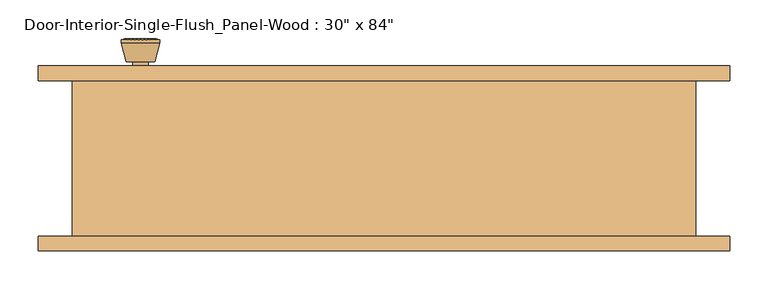
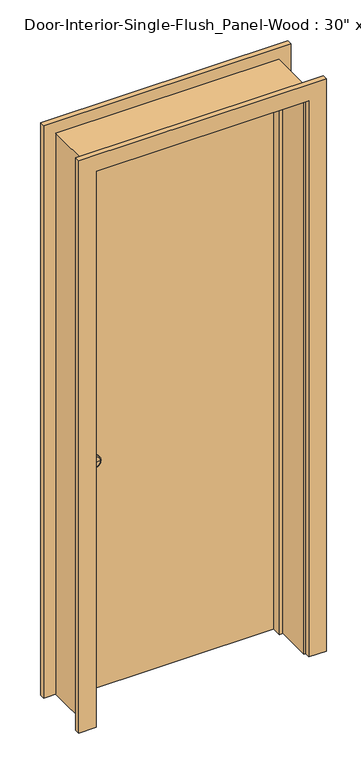
"""IFC4 building model written with IfcOpenShell, lengths in millimetres: door geometry."""

from ifc_helpers import new_model, si_unit, point, frame, frame_2d, origin, origin_with_axes, place, context, project, spatial, polyline, circle_curve, trimmed, segment, composite_curve, outline, extrude, faceted_brep, source, transform, mapped, element, save
from ifc_brep_helpers import plane_surface, cylinder_surface, revolved_surface, advanced_brep


def door_715cd483(model_context):
    return source(origin(), model_context, "Body", "SolidModel", [
        advanced_brep(
        [(-317.5, 57.5, 914.4), (-307.5, 57.5, 914.4), (-327.5, 57.5, 914.4), (-297.0241324, 8.5, 914.4), (-317.5, 8.5, 914.4), (-337.9758676, 8.5, 914.4), (-292.5, 10.3278681, 914.4), (-342.5, 10.3278681, 914.4), (-292.5, 13.7915463, 914.4), (-342.5, 13.7915463, 914.4), (-298.863764, 38.5, 914.4), (-336.136236, 38.5, 914.4), (-307.5, 38.5, 914.4), (-327.5, 38.5, 914.4)],
        [
            (0, 1),
            (1, 2, circle_curve(frame((-317.5, 57.5, 914.4), z_axis=(0.0, 1.0, 0.0), x_axis=(-1.0, 0.0, 0.0)), 10.0)),
            (2, 0),
            (2, 1, circle_curve(frame((-317.5, 57.5, 914.4), z_axis=(0.0, 1.0, 0.0), x_axis=(-1.0, 0.0, 0.0)), 10.0)),
            (3, 4),
            (4, 5),
            (5, 3, circle_curve(frame((-317.5, 8.5, 914.4), z_axis=(0.0, -1.0, 0.0), x_axis=(-1.0, 0.0, 0.0)), 20.4758676)),
            (3, 5, circle_curve(frame((-317.5, 8.5, 914.4), z_axis=(0.0, -1.0, 0.0), x_axis=(-1.0, 0.0, 0.0)), 20.4758676)),
            (6, 3),
            (5, 7),
            (7, 6, circle_curve(frame((-317.5, 10.3278681, 914.4), z_axis=(0.0, -1.0, 0.0), x_axis=(-1.0, 0.0, 0.0)), 25.0)),
            (6, 7, circle_curve(frame((-317.5, 10.3278681, 914.4), z_axis=(0.0, -1.0, 0.0), x_axis=(-1.0, 0.0, 0.0)), 25.0)),
            (8, 6),
            (7, 9),
            (9, 8, circle_curve(frame((-317.5, 13.7915463, 914.4), z_axis=(0.0, -1.0, 0.0), x_axis=(-1.0, 0.0, 0.0)), 25.0)),
            (8, 9, circle_curve(frame((-317.5, 13.7915463, 914.4), z_axis=(0.0, -1.0, 0.0), x_axis=(-1.0, 0.0, 0.0)), 25.0)),
            (10, 8),
            (9, 11),
            (11, 10, circle_curve(frame((-317.5, 38.5, 914.4), z_axis=(0.0, -1.0, 0.0), x_axis=(-1.0, 0.0, 0.0)), 18.636236)),
            (10, 11, circle_curve(frame((-317.5, 38.5, 914.4), z_axis=(0.0, -1.0, 0.0), x_axis=(-1.0, 0.0, 0.0)), 18.636236)),
            (12, 10),
            (11, 13),
            (13, 12, circle_curve(frame((-317.5, 38.5, 914.4), z_axis=(0.0, -1.0, 0.0), x_axis=(-1.0, 0.0, 0.0)), 10.0)),
            (12, 13, circle_curve(frame((-317.5, 38.5, 914.4), z_axis=(0.0, -1.0, 0.0), x_axis=(-1.0, 0.0, 0.0)), 10.0)),
            (1, 12),
            (13, 2),
        ],
        [
            plane_surface(frame((-317.5, 57.5, 914.4), z_axis=(0.0, 1.0, 0.0), x_axis=(-1.0, 0.0, 0.0))),
            plane_surface(frame((-317.5, 8.5, 914.4), z_axis=(0.0, -1.0, 0.0), x_axis=(-1.0, 0.0, 0.0))),
            revolved_surface(polyline([(-337.9758676, 8.5, 914.4), (-342.5, 10.3278681, 914.4)]), (-317.5, 57.5, 914.4), (0.0, 1.0, 0.0)),
            cylinder_surface(frame((-317.5, 57.5, 914.4), z_axis=(0.0, 1.0, 0.0), x_axis=(-1.0, 0.0, 0.0)), 25.0),
            revolved_surface(polyline([(-342.5, 13.7915463, 914.4), (-336.136236, 38.5, 914.4)]), (-317.5, 57.5, 914.4), (0.0, 1.0, 0.0)),
            plane_surface(frame((-317.5, 38.5, 914.4), z_axis=(0.0, 1.0, 0.0), x_axis=(-1.0, 0.0, 0.0))),
            cylinder_surface(frame((-317.5, 57.5, 914.4), z_axis=(0.0, 1.0, 0.0), x_axis=(-1.0, 0.0, 0.0)), 10.0),
        ],
        [
            (0, [[1, 2, 3]]),
            (0, [[-3, 4, -1]]),
            (1, [[5, 6, 7]]),
            (1, [[-6, -5, 8]]),
            (2, [[9, -7, 10, 11]]),
            (2, [[-10, -8, -9, 12]]),
            (3, [[13, -11, 14, 15]]),
            (3, [[-14, -12, -13, 16]]),
            (4, [[17, -15, 18, 19]]),
            (4, [[-18, -16, -17, 20]]),
            (5, [[21, -19, 22, 23]]),
            (5, [[-22, -20, -21, 24]]),
            (6, [[25, -23, 26, -2]]),
            (6, [[-26, -24, -25, -4]]),
        ],
    ),
        extrude(outline(composite_curve([segment(trimmed(circle_curve(frame_2d((914.4, -317.5)), 30.0), [point((914.4, -347.5))], [point((914.4, -287.5))], False, "CARTESIAN"), True, "CONTINUOUS"), segment(trimmed(circle_curve(frame_2d((914.4, -317.5)), 30.0), [point((914.4, -287.5))], [point((914.4, -347.5))], False, "CARTESIAN"), True, "CONTINUOUS")], self_intersect=False)), frame((0.0, 57.5, 0.0), z_axis=(0.0, 1.0, 0.0), x_axis=(0.0, 0.0, 1.0)), (0.0, 0.0, 1.0), 6.0),
        advanced_brep(
        [(-317.5, 104.425, 914.4), (-327.5, 104.425, 914.4), (-307.5, 104.425, 914.4), (-297.0241324, 153.425, 914.4), (-337.9758676, 153.425, 914.4), (-317.5, 153.425, 914.4), (-292.5, 151.5971319, 914.4), (-342.5, 151.5971319, 914.4), (-292.5, 148.1334537, 914.4), (-342.5, 148.1334537, 914.4), (-298.863764, 123.425, 914.4), (-336.136236, 123.425, 914.4), (-307.5, 123.425, 914.4), (-327.5, 123.425, 914.4)],
        [
            (0, 1),
            (1, 2, circle_curve(frame((-317.5, 104.425, 914.4), z_axis=(0.0, -1.0, 0.0), x_axis=(-1.0, 0.0, 0.0)), 10.0)),
            (2, 0),
            (2, 1, circle_curve(frame((-317.5, 104.425, 914.4), z_axis=(0.0, -1.0, 0.0), x_axis=(-1.0, 0.0, 0.0)), 10.0)),
            (3, 4, circle_curve(frame((-317.5, 153.425, 914.4), z_axis=(0.0, 1.0, 0.0), x_axis=(-1.0, 0.0, 0.0)), 20.4758676)),
            (4, 5),
            (5, 3),
            (4, 3, circle_curve(frame((-317.5, 153.425, 914.4), z_axis=(0.0, 1.0, 0.0), x_axis=(-1.0, 0.0, 0.0)), 20.4758676)),
            (6, 7, circle_curve(frame((-317.5, 151.5971319, 914.4), z_axis=(0.0, 1.0, 0.0), x_axis=(-1.0, 0.0, 0.0)), 25.0)),
            (7, 4),
            (3, 6),
            (7, 6, circle_curve(frame((-317.5, 151.5971319, 914.4), z_axis=(0.0, 1.0, 0.0), x_axis=(-1.0, 0.0, 0.0)), 25.0)),
            (8, 9, circle_curve(frame((-317.5, 148.1334537, 914.4), z_axis=(0.0, 1.0, 0.0), x_axis=(-1.0, 0.0, 0.0)), 25.0)),
            (9, 7),
            (6, 8),
            (9, 8, circle_curve(frame((-317.5, 148.1334537, 914.4), z_axis=(0.0, 1.0, 0.0), x_axis=(-1.0, 0.0, 0.0)), 25.0)),
            (10, 11, circle_curve(frame((-317.5, 123.425, 914.4), z_axis=(0.0, 1.0, 0.0), x_axis=(-1.0, 0.0, 0.0)), 18.636236)),
            (11, 9),
            (8, 10),
            (11, 10, circle_curve(frame((-317.5, 123.425, 914.4), z_axis=(0.0, 1.0, 0.0), x_axis=(-1.0, 0.0, 0.0)), 18.636236)),
            (12, 13, circle_curve(frame((-317.5, 123.425, 914.4), z_axis=(0.0, 1.0, 0.0), x_axis=(-1.0, 0.0, 0.0)), 10.0)),
            (13, 11),
            (10, 12),
            (13, 12, circle_curve(frame((-317.5, 123.425, 914.4), z_axis=(0.0, 1.0, 0.0), x_axis=(-1.0, 0.0, 0.0)), 10.0)),
            (1, 13),
            (12, 2),
        ],
        [
            plane_surface(frame((-317.5, 104.425, 914.4), z_axis=(0.0, -1.0, 0.0), x_axis=(-1.0, 0.0, 0.0))),
            plane_surface(frame((-317.5, 153.425, 914.4), z_axis=(0.0, 1.0, 0.0), x_axis=(-1.0, 0.0, 0.0))),
            revolved_surface(polyline([(-337.9758676, 153.425, 914.4), (-342.5, 151.5971319, 914.4)]), (-317.5, 104.425, 914.4), (0.0, -1.0, 0.0)),
            cylinder_surface(frame((-317.5, 104.425, 914.4), z_axis=(0.0, -1.0, 0.0), x_axis=(-1.0, 0.0, 0.0)), 25.0),
            revolved_surface(polyline([(-342.5, 148.1334537, 914.4), (-336.136236, 123.425, 914.4)]), (-317.5, 104.425, 914.4), (0.0, -1.0, 0.0)),
            plane_surface(frame((-317.5, 123.425, 914.4), z_axis=(0.0, -1.0, 0.0), x_axis=(-1.0, 0.0, 0.0))),
            cylinder_surface(frame((-317.5, 104.425, 914.4), z_axis=(0.0, -1.0, 0.0), x_axis=(-1.0, 0.0, 0.0)), 10.0),
        ],
        [
            (0, [[1, 2, 3]]),
            (0, [[-3, 4, -1]]),
            (1, [[5, 6, 7]]),
            (1, [[8, -7, -6]]),
            (2, [[9, 10, -5, 11]]),
            (2, [[12, -11, -8, -10]]),
            (3, [[13, 14, -9, 15]]),
            (3, [[16, -15, -12, -14]]),
            (4, [[17, 18, -13, 19]]),
            (4, [[20, -19, -16, -18]]),
            (5, [[21, 22, -17, 23]]),
            (5, [[24, -23, -20, -22]]),
            (6, [[-2, 25, -21, 26]]),
            (6, [[-4, -26, -24, -25]]),
        ],
    ),
        extrude(outline(composite_curve([segment(trimmed(circle_curve(frame_2d((914.4, -317.5)), 30.0), [point((914.4, -347.5))], [point((914.4, -287.5))], False, "CARTESIAN"), True, "CONTINUOUS"), segment(trimmed(circle_curve(frame_2d((914.4, -317.5)), 30.0), [point((914.4, -287.5))], [point((914.4, -347.5))], False, "CARTESIAN"), True, "CONTINUOUS")], self_intersect=False)), frame((0.0, 98.425, 0.0), z_axis=(0.0, 1.0, 0.0), x_axis=(0.0, 0.0, 1.0)), (0.0, 0.0, 1.0), 6.0),
        extrude(outline(polyline([(381.0, 63.5), (-381.0, 63.5), (-381.0, 98.425), (381.0, 98.425), (381.0, 63.5)])), origin_with_axes(), (0.0, 0.0, 1.0), 2133.6),
        faceted_brep([(406.4, 98.425, 0.0), (406.4, -104.775, 0.0), (381.0, -104.775, 0.0), (381.0, 28.575, 0.0), (368.3, 28.575, 0.0), (368.3, 63.5, 0.0), (381.0, 63.5, 0.0), (381.0, 98.425, 0.0), (406.4, 98.425, 2159.0), (406.4, -104.775, 2159.0), (-406.4, -104.775, 2159.0), (-406.4, -104.775, 0.0), (-381.0, -104.775, 0.0), (-381.0, -104.775, 2133.6), (381.0, -104.775, 2133.6), (381.0, 28.575, 2133.6), (-381.0, 28.575, 2133.6), (-381.0, 28.575, 0.0), (-368.3, 28.575, 0.0), (-368.3, 28.575, 2120.9), (368.3, 28.575, 2120.9), (368.3, 63.5, 2120.9), (-368.3, 63.5, 2120.9), (-368.3, 63.5, 0.0), (-381.0, 63.5, 0.0), (-381.0, 63.5, 2133.6), (381.0, 63.5, 2133.6), (381.0, 98.425, 2133.6), (-381.0, 98.425, 2133.6), (-381.0, 98.425, 0.0), (-406.4, 98.425, 0.0), (-406.4, 98.425, 2159.0)], [[[0, 1, 2, 3, 4, 5, 6, 7]], [[1, 0, 8, 9]], [[2, 1, 9, 10, 11, 12, 13, 14]], [[3, 2, 14, 15]], [[4, 3, 15, 16, 17, 18, 19, 20]], [[5, 4, 20, 21]], [[6, 5, 21, 22, 23, 24, 25, 26]], [[7, 6, 26, 27]], [[0, 7, 27, 28, 29, 30, 31, 8]], [[9, 8, 31, 10]], [[15, 14, 13, 16]], [[21, 20, 19, 22]], [[27, 26, 25, 28]], [[30, 29, 24, 23, 18, 17, 12, 11]], [[10, 31, 30, 11]], [[16, 13, 12, 17]], [[22, 19, 18, 23]], [[28, 25, 24, 29]]]),
        extrude(outline(polyline([(0.0, 387.35), (0.0, 450.85), (2203.45, 450.85), (2203.45, -450.85), (0.0, -450.85), (0.0, -387.35), (2139.95, -387.35), (2139.95, 387.35), (0.0, 387.35)])), frame((0.0, -123.825, 0.0), z_axis=(0.0, 1.0, 0.0), x_axis=(0.0, 0.0, 1.0)), (0.0, 0.0, 1.0), 19.05),
        extrude(outline(polyline([(0.0, 387.35), (0.0, 450.85), (2203.45, 450.85), (2203.45, -450.85), (0.0, -450.85), (0.0, -387.35), (2139.95, -387.35), (2139.95, 387.35), (0.0, 387.35)])), frame((0.0, 98.425, 0.0), z_axis=(0.0, 1.0, 0.0), x_axis=(0.0, 0.0, 1.0)), (0.0, 0.0, 1.0), 19.05),
    ])


if __name__ == "__main__":
    model = new_model("IFC4")
    model_context = context("Model", 3, world=origin())
    ifc_project = project(units=[si_unit("LENGTHUNIT", "METRE", prefix="MILLI")], contexts=[model_context])
    site = spatial("IfcSite", under=ifc_project)
    building = spatial("IfcBuilding", under=site)
    placement = place(None, origin())
    door_shape = door_715cd483(model_context)
    element("IfcDoor", 1, ObjectType="Door-Interior-Single-Flush_Panel-Wood : 30\" x 84\"", at=placement, inside=building, context=model_context, shape_type="MappedRepresentation", body=[
        mapped(door_shape, transform((0.0, 0.0, 0.0), x_axis=(1.0, 0.0, 0.0), y_axis=(0.0, 1.0, 0.0), z_axis=(0.0, 0.0, 1.0))),
    ])
    save(model, "model.ifc")

# Revit data of these elements
# Type "Door-Interior-Single-Flush_Panel-Wood : 30\" x 84\""
#   Type Mark = "12"
#   Assembly Code = "C1020300"
#   Analytic Construction = "Wooden"
#   Thickness = 0' - 1 3/8"
#   Thermal Resistance (R) = 2.5876 (h·ft²·°F)/BTU
#   Swing Angle [instance default] = 90.00°
#   Rough Width = 2' - 8"
#   Rough Height = 7' - 1"
#   Height = 7' - 0"
#   Width = 2' - 6"
#   Heat Transfer Coefficient (U) = 0.3865 BTU/(h·ft²·°F)
#   Trim Material = Cherry
#   Panel Material = Cherry
#   Frame Material = Cherry
#   Door Handle Material = Aluminum
#   Visual Light Transmittance = 0
#   Solar Heat Gain Coefficient = 0
#   Wall Closure = (empty or 0)
#   Function = (empty or 0)
# Element 1 (IfcDoor, "Door-Interior-Single-Flush_Panel-Wood : 30\" x 84\"")
#   Materials on its faces: "Cherry", "Aluminum"
# Materials
#   "Cherry": class "Wood", colour RGB 226 177 128, transparency 0, Description = "Prunus Serotina", Cost = 0
#   "Aluminum": class "Metal", colour RGB 247 247 247, transparency 0, Description = "Aluminum 6061", Cost = 0
